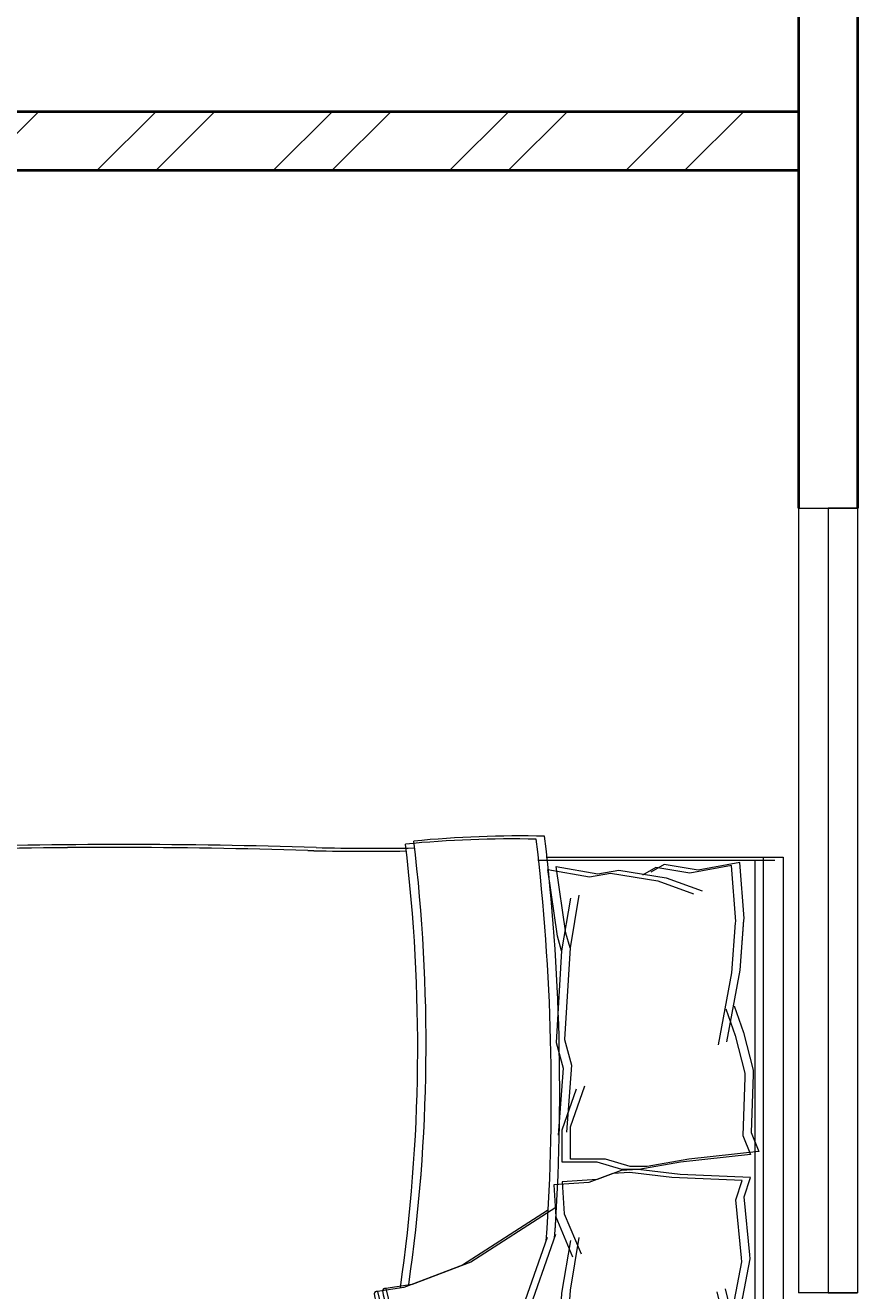
# Model space of a CAD drawing. Units: inches. Extents: x 1601 to 2297, y 1496 to 2631.
# Tile 48 of 57: x 2167 to 2231, y 2141 to 2237. Entities that reach past the tile are written whole.
import ezdxf

# ---------------------------------------------------------------- set-up
doc = ezdxf.new("R2010")
doc.units = ezdxf.units.IN
for name, color, linetype, lineweight in [('A-ANNO-DIMS', 2, 'Continuous', 18), ('A-FURN', 8, 'Continuous', 18), ('A-GLAZ', 161, 'Continuous', 20), ('A-WALL', 7, 'Continuous', 40), ('A-WALL-PATT', 215, 'Continuous', 13)]:
    doc.layers.add(name, color=color, linetype=linetype, lineweight=lineweight)
doc.styles.get("Standard").update_dxf_attribs({"font": 'arial.ttf'})
doc.dimstyles.get("Standard").update_dxf_attribs({"dimtxt": 0.18, "dimasz": 0.18, "dimexe": 0.18, "dimexo": 0.0625, "dimgap": 0.09, "dimtad": 0, "dimtih": 1, "dimtoh": 1, "dimdec": 4, "dimzin": 0, "dimdsep": 46, "dimtxsty": 'Standard', "dimcen": 0.09, "dimadec": 0, "dimazin": 0, "dimtfac": 1, "dimtdec": 4, "dimtofl": 0, "dimtmove": 0, "dimatfit": 3, "dimfxl": 1, "dimtolj": 1, "dimtzin": 0, "dimarcsym": 0})

# ---------------------------------------------------------------- blocks, each defined once
blk = doc.blocks.new('BED-DOUBLE')
for p, q in [((27.746, 52.867), (24.495, 49.162)), ((27.746, 52.867), (24.495, 49.162)), ((27.746, 52.867), (24.495, 49.162)), ((27.746, 52.867), (24.495, 49.162)), ((28.385, 53.096), (25.135, 49.39)), ((28.385, 53.096), (25.135, 49.39)), ((28.385, 53.096), (25.135, 49.39)), ((28.385, 53.096), (25.135, 49.39)), ((29.49, 52.947), (27.746, 52.867, 3.871)), ((29.49, 52.947), (27.746, 52.867, 3.871)), ((29.49, 52.947), (27.746, 52.867, 3.871)), ((29.49, 52.947), (27.746, 52.867, 3.871)), ((28.365, 51.33), (27.746, 52.867)), ((28.365, 51.33), (27.746, 52.867)), ((28.365, 51.33), (27.746, 52.867)), ((28.365, 51.33), (27.746, 52.867)), ((30.13, 53.175), (28.385, 53.096, 3.871)), ((30.13, 53.175), (28.385, 53.096, 3.871)), ((30.13, 53.175), (28.385, 53.096, 3.871)), ((30.13, 53.175), (28.385, 53.096, 3.871)), ((29.004, 51.559), (28.385, 53.096)), ((29.004, 51.558), (28.385, 53.096)), ((29.004, 51.559), (28.385, 53.096)), ((29.004, 51.558), (28.385, 53.096)), ((0, 51.494), (0.639, 51.493)), ((0, 3.475), (0, 51.494)), ((0, 51.494), (0.639, 51.493)), ((0, 3.475), (0, 51.494)), ((0.639, 51.494), (27.249, 51.494)), ((0.639, 51.494), (27.249, 51.494)), ((0.639, 51.493), (27.249, 51.493)), ((0.639, 51.493), (27.249, 51.493)), ((2.173, 3.703), (2.173, 51.494)), ((2.173, 3.703), (2.173, 51.494)), ((2.173, 3.703), (2.173, 51.493)), ((2.173, 3.703), (2.173, 51.493)), ((28.055, 48.233), (28.365, 51.33)), ((28.055, 48.233), (28.365, 51.33)), ((28.055, 48.233), (28.365, 51.33)), ((28.055, 48.233), (28.365, 51.33)), ((28.695, 48.461), (29.004, 51.559)), ((28.695, 48.461), (29.004, 51.559)), ((28.695, 48.461), (29.004, 51.558)), ((28.695, 48.461), (29.004, 51.558)), ((0, 51.265), (26.61, 51.265)), ((0, 51.265), (26.61, 51.265)), ((0, 51.265), (26.61, 51.265)), ((0, 51.265), (26.61, 51.265)), ((1.533, 3.475), (1.533, 51.265)), ((1.533, 3.475), (1.533, 51.265)), ((1.533, 3.475), (1.533, 51.265)), ((1.533, 3.475), (1.533, 51.265)), ((3.196, 50.34), (3.099, 44.938)), ((3.196, 50.34), (3.099, 44.938)), ((3.196, 50.34), (3.099, 44.938)), ((3.196, 50.34), (3.099, 44.938)), ((3.196, 50.34), (6.407, 49.961)), ((3.196, 50.34), (6.407, 49.961)), ((3.196, 50.34), (6.407, 49.961)), ((3.196, 50.34), (6.407, 49.961)), ((5.768, 49.733), (8.338, 50.328)), ((5.768, 49.733), (8.338, 50.328)), ((5.768, 49.733), (8.338, 50.328)), ((5.768, 49.733), (8.338, 50.328)), ((6.407, 49.961), (8.977, 50.557)), ((6.407, 49.961), (8.977, 50.557)), ((6.407, 49.961), (8.977, 50.556)), ((6.407, 49.961), (8.977, 50.556)), ((8.338, 50.328), (9.384, 49.814)), ((8.338, 50.328), (9.384, 49.814)), ((8.338, 50.328), (9.384, 49.814)), ((8.338, 50.328), (9.384, 49.814)), ((12.468, 50.34), (8.896, 49.538)), ((12.468, 50.34), (8.896, 49.537)), ((12.468, 50.34), (8.896, 49.538)), ((12.468, 50.34), (8.896, 49.537)), ((8.977, 50.557), (10.024, 50.043)), ((8.977, 50.557), (10.024, 50.043)), ((8.977, 50.556), (10.024, 50.042)), ((8.977, 50.556), (10.024, 50.042)), ((14.073, 50.151), (12.468, 50.34)), ((14.073, 50.151), (12.468, 50.34)), ((14.073, 50.151), (12.468, 50.34)), ((14.073, 50.151), (12.468, 50.34)), ((16.573, 50.698), (13.434, 49.923)), ((16.573, 50.698), (13.434, 49.922)), ((16.573, 50.698), (13.434, 49.923)), ((16.573, 50.698), (13.434, 49.922)), ((17.212, 50.926), (14.073, 50.151)), ((17.212, 50.926), (14.073, 50.151)), ((17.212, 50.926), (14.073, 50.151)), ((17.212, 50.926), (14.073, 50.151)), ((16.169, 45.566), (16.573, 50.698)), ((16.169, 45.566), (16.573, 50.698)), ((16.169, 45.566), (16.573, 50.698)), ((16.169, 45.566), (16.573, 50.698)), ((16.808, 45.795), (17.212, 50.926)), ((16.808, 45.794), (17.212, 50.926)), ((16.808, 45.795), (17.212, 50.926)), ((16.808, 45.794), (17.212, 50.926)), ((2.557, 50.112), (2.46, 44.709)), ((2.557, 50.112), (2.46, 44.709)), ((2.557, 50.111), (2.46, 44.709)), ((2.557, 50.111), (2.46, 44.709)), ((2.557, 50.112), (5.768, 49.733)), ((2.557, 50.112), (5.768, 49.733)), ((2.557, 50.111), (5.768, 49.733)), ((2.557, 50.111), (5.768, 49.733)), ((8.896, 49.538), (6.218, 48.356)), ((8.896, 49.538), (6.218, 48.356)), ((8.896, 49.537), (6.218, 48.356)), ((8.896, 49.537), (6.218, 48.356)), ((11.829, 50.112), (8.257, 49.309)), ((11.829, 50.112), (8.257, 49.309)), ((11.829, 50.112), (8.257, 49.309)), ((11.829, 50.112), (8.257, 49.309)), ((13.434, 49.923), (11.829, 50.112)), ((13.434, 49.922), (11.829, 50.112)), ((13.434, 49.923), (11.829, 50.112)), ((13.434, 49.922), (11.829, 50.112)), ((25.135, 49.39), (22.968, 46.448)), ((25.135, 49.39), (22.968, 46.448)), ((25.135, 49.39), (22.968, 46.448)), ((25.135, 49.39), (22.968, 46.448)), ((8.257, 49.309), (5.578, 48.128)), ((8.257, 49.309), (5.578, 48.128)), ((8.257, 49.309), (5.578, 48.128)), ((8.257, 49.309), (5.578, 48.128)), ((24.495, 49.162), (22.329, 46.219)), ((24.495, 49.162), (22.329, 46.219)), ((24.495, 49.162), (22.329, 46.219)), ((24.495, 49.162), (22.329, 46.219)), ((29.004, 44.589), (28.695, 48.461)), ((29.004, 44.589), (28.695, 48.461)), ((29.004, 44.589), (28.695, 48.461)), ((29.004, 44.589), (28.695, 48.461)), ((28.365, 44.361), (28.055, 48.233)), ((28.365, 44.361), (28.055, 48.233)), ((28.365, 44.361), (28.055, 48.233)), ((28.365, 44.361), (28.055, 48.233)), ((22.968, 46.448), (20.956, 40.872)), ((22.968, 46.448), (20.956, 40.872)), ((22.968, 46.448), (20.956, 40.872)), ((22.968, 46.448), (20.956, 40.872)), ((2.46, 44.709), (2.542, 45.712)), ((2.46, 44.709), (2.542, 45.712)), ((2.46, 44.709), (2.542, 45.712)), ((2.46, 44.709), (2.542, 45.712)), ((2.542, 45.712), (3.069, 41.914)), ((2.542, 45.712), (3.069, 41.914)), ((2.542, 45.712), (3.069, 41.914)), ((2.542, 45.712), (3.069, 41.914)), ((3.099, 44.938), (3.181, 45.941)), ((3.099, 44.938), (3.181, 45.941)), ((3.099, 44.938), (3.181, 45.94)), ((3.099, 44.938), (3.181, 45.94)), ((3.181, 45.941), (3.709, 42.143)), ((3.181, 45.941), (3.709, 42.143)), ((3.181, 45.94), (3.709, 42.142)), ((3.181, 45.94), (3.709, 42.142)), ((16.726, 43.606), (16.169, 45.566)), ((16.726, 43.606), (16.169, 45.566)), ((16.726, 43.606), (16.169, 45.566)), ((16.726, 43.606), (16.169, 45.566)), ((17.365, 43.834), (16.808, 45.795)), ((17.365, 43.834), (16.808, 45.795)), ((17.365, 43.834), (16.808, 45.794)), ((17.365, 43.834), (16.808, 45.794)), ((22.329, 46.219), (20.316, 40.644)), ((22.329, 46.219), (20.316, 40.644)), ((22.329, 46.219), (20.317, 40.644)), ((22.329, 46.219), (20.317, 40.644)), ((29.468, 41.182), (29.004, 44.589)), ((29.469, 41.182), (29.004, 44.589)), ((29.468, 41.182), (29.004, 44.589)), ((29.469, 41.182), (29.004, 44.589)), ((16.295, 36.596), (16.726, 43.606)), ((16.295, 36.596), (16.726, 43.606)), ((16.295, 36.596), (16.726, 43.606)), ((16.295, 36.596), (16.726, 43.606)), ((16.934, 36.824), (17.365, 43.834)), ((16.934, 36.824), (17.365, 43.834)), ((16.934, 36.824), (17.365, 43.834)), ((16.934, 36.824), (17.365, 43.834)), ((28.829, 40.954), (28.365, 44.361)), ((28.829, 40.953), (28.365, 44.361)), ((28.829, 40.954), (28.365, 44.361)), ((28.829, 40.953), (28.365, 44.361)), ((3.069, 41.914), (4.422, 36.495)), ((3.069, 41.914), (4.422, 36.495)), ((3.069, 41.914), (4.422, 36.495)), ((3.069, 41.914), (4.422, 36.495)), ((3.709, 42.143), (5.061, 36.723)), ((3.709, 42.143), (5.061, 36.723)), ((3.709, 42.142), (5.061, 36.723)), ((3.709, 42.142), (5.061, 36.723)), ((20.316, 40.644), (17.383, 32.306)), ((20.317, 40.644), (17.383, 32.306)), ((20.316, 40.644), (17.383, 32.306)), ((20.317, 40.644), (17.383, 32.306)), ((20.956, 40.872), (18.022, 32.534)), ((20.956, 40.872), (18.022, 32.534)), ((20.956, 40.872), (18.022, 32.534)), ((20.956, 40.872), (18.022, 32.534)), ((29.758, 38.94), (28.829, 40.954)), ((29.758, 38.94), (28.829, 40.954)), ((29.758, 38.94), (28.829, 40.953)), ((29.758, 38.94), (28.829, 40.953)), ((30.397, 39.169), (29.468, 41.182)), ((30.397, 39.169), (29.468, 41.182)), ((30.397, 39.168), (29.469, 41.182)), ((30.397, 39.168), (29.469, 41.182)), ((79.245, 15.063), (79.245, 39.677)), ((79.245, 15.063), (79.245, 39.677)), ((79.245, 15.063), (79.245, 39.677)), ((79.245, 15.063), (79.245, 39.677)), ((79.884, 15.292), (79.884, 39.905)), ((79.884, 15.291), (79.884, 39.905)), ((79.884, 15.292), (79.884, 39.905)), ((79.884, 15.291), (79.884, 39.905)), ((3.673, 39.2), (3.078, 37.135)), ((3.673, 39.2), (3.078, 37.135)), ((3.673, 39.2), (3.078, 37.135)), ((3.673, 39.2), (3.078, 37.135)), ((4.313, 39.428), (3.717, 37.363)), ((4.313, 39.428), (3.717, 37.363)), ((4.313, 39.428), (3.718, 37.363)), ((4.313, 39.428), (3.718, 37.363)), ((30.377, 36.462), (29.758, 38.94)), ((30.377, 36.462), (29.758, 38.94)), ((30.377, 36.462), (29.758, 38.94)), ((30.377, 36.462), (29.758, 38.94)), ((31.016, 36.691), (30.397, 39.169)), ((31.016, 36.691), (30.397, 39.169)), ((31.016, 36.691), (30.397, 39.168)), ((31.016, 36.691), (30.397, 39.168)), ((3.078, 37.135), (2.537, 34.204)), ((3.078, 37.135), (2.537, 34.204)), ((3.078, 37.135), (2.537, 34.204)), ((3.078, 37.135), (2.537, 34.204)), ((3.717, 37.363), (3.176, 34.433)), ((3.718, 37.363), (3.176, 34.433)), ((3.717, 37.363), (3.176, 34.433)), ((3.718, 37.363), (3.176, 34.433)), ((16.268, 32.792), (16.934, 36.824)), ((16.268, 32.792), (16.934, 36.824)), ((16.268, 32.792), (16.934, 36.824)), ((16.268, 32.792), (16.934, 36.824)), ((15.628, 32.564), (16.295, 36.596)), ((15.628, 32.564), (16.295, 36.596)), ((15.628, 32.564), (16.295, 36.596)), ((15.628, 32.564), (16.295, 36.596)), ((23.876, 34.449), (28.365, 36.153)), ((23.876, 34.449), (28.365, 36.153)), ((23.876, 34.449), (28.365, 36.152)), ((23.876, 34.449), (28.365, 36.152)), ((24.516, 34.677), (29.004, 36.381)), ((24.516, 34.677), (29.004, 36.381)), ((24.516, 34.677), (29.004, 36.381)), ((24.516, 34.677), (29.004, 36.381)), ((28.365, 36.153), (30.377, 36.462)), ((28.365, 36.152), (30.377, 36.462)), ((28.365, 36.153), (30.377, 36.462)), ((28.365, 36.152), (30.377, 36.462)), ((29.004, 36.381), (31.016, 36.691)), ((29.004, 36.381), (31.016, 36.691)), ((29.004, 36.381), (31.016, 36.691)), ((29.004, 36.381), (31.016, 36.691)), ((2.537, 34.204), (2.557, 33.883)), ((2.537, 34.204), (2.557, 33.883)), ((2.537, 34.204), (2.557, 33.883)), ((2.537, 34.204), (2.557, 33.883)), ((2.557, 33.883), (2.979, 29.456)), ((2.557, 33.883), (2.979, 29.455)), ((2.557, 33.883), (2.979, 29.456)), ((2.557, 33.883), (2.979, 29.455)), ((3.176, 34.433), (3.196, 34.112)), ((3.176, 34.433), (3.196, 34.112)), ((3.176, 34.433), (3.196, 34.112)), ((3.176, 34.433), (3.196, 34.112)), ((3.196, 34.112), (3.618, 29.684)), ((3.196, 34.112), (3.618, 29.684)), ((3.196, 34.112), (3.618, 29.684)), ((3.196, 34.112), (3.618, 29.684)), ((17.379, 30.978), (16.094, 34.049)), ((17.379, 30.978), (16.094, 34.049)), ((17.379, 30.978), (16.094, 34.049)), ((17.379, 30.978), (16.094, 34.049)), ((17.383, 30.259), (23.876, 34.449)), ((17.383, 30.259), (23.876, 34.449)), ((17.383, 30.259), (23.876, 34.449)), ((17.383, 30.259), (23.876, 34.449)), ((18.022, 30.487), (24.516, 34.677)), ((18.022, 30.487), (24.516, 34.677)), ((18.022, 30.487), (24.516, 34.677)), ((18.022, 30.487), (24.516, 34.677)), ((16.739, 30.75), (15.454, 33.821)), ((16.739, 30.75), (15.454, 33.821)), ((16.739, 30.75), (15.454, 33.82)), ((16.739, 30.75), (15.454, 33.82)), ((17.532, 28.526), (17.379, 30.978)), ((17.532, 28.525), (17.379, 30.978)), ((17.532, 28.526), (17.379, 30.978)), ((17.532, 28.525), (17.379, 30.978)), ((16.893, 28.297), (16.739, 30.75)), ((16.893, 28.297), (16.739, 30.75)), ((16.893, 28.297), (16.739, 30.75)), ((16.893, 28.297), (16.739, 30.75)), ((2.979, 29.456), (2.492, 27.977)), ((2.979, 29.456), (2.492, 27.977)), ((2.979, 29.455), (2.492, 27.976)), ((2.979, 29.455), (2.492, 27.976)), ((3.618, 29.684), (3.131, 28.205)), ((3.618, 29.684), (3.131, 28.205)), ((3.618, 29.684), (3.131, 28.205)), ((3.618, 29.684), (3.131, 28.205)), ((3.131, 28.205), (8.506, 27.962)), ((3.131, 28.205), (8.506, 27.961)), ((3.131, 28.205), (8.506, 27.962)), ((3.131, 28.205), (8.506, 27.961)), ((12.377, 27.436), (14.216, 28.13)), ((12.377, 27.436), (14.217, 28.13)), ((12.377, 27.436), (14.216, 28.13)), ((12.377, 27.436), (14.217, 28.13)), ((13.016, 27.664), (14.856, 28.359)), ((13.016, 27.664), (14.856, 28.359)), ((13.016, 27.664), (14.856, 28.358)), ((13.016, 27.664), (14.856, 28.358)), ((14.216, 28.13), (16.893, 28.297)), ((14.216, 28.13), (16.893, 28.297)), ((14.217, 28.13), (16.893, 28.297)), ((14.217, 28.13), (16.893, 28.297)), ((14.856, 28.359), (17.532, 28.526)), ((14.856, 28.359), (17.532, 28.526)), ((14.856, 28.358), (17.532, 28.525)), ((14.856, 28.358), (17.532, 28.525)), ((2.492, 27.977), (7.867, 27.733)), ((2.492, 27.977), (7.867, 27.733)), ((2.492, 27.976), (7.867, 27.733)), ((2.492, 27.976), (7.867, 27.733)), ((7.22, 26.561), (10.401, 27.139)), ((7.22, 26.56), (10.401, 27.139)), ((7.22, 26.561), (10.401, 27.139)), ((7.22, 26.56), (10.401, 27.139)), ((7.859, 26.789), (11.04, 27.367)), ((7.859, 26.789), (11.04, 27.367)), ((7.859, 26.789), (11.04, 27.367)), ((7.859, 26.789), (11.04, 27.367)), ((7.867, 27.733), (11.078, 27.355)), ((7.867, 27.733), (11.078, 27.354)), ((7.867, 27.733), (11.078, 27.355)), ((7.867, 27.733), (11.078, 27.354)), ((8.506, 27.962), (11.717, 27.583)), ((8.506, 27.962), (11.717, 27.583)), ((8.506, 27.961), (11.717, 27.583)), ((8.506, 27.961), (11.717, 27.583)), ((10.401, 27.139), (11.702, 27.139)), ((10.401, 27.139), (11.702, 27.139)), ((10.401, 27.139), (11.702, 27.139)), ((10.401, 27.139), (11.702, 27.139)), ((11.04, 27.367), (12.341, 27.367)), ((11.04, 27.367), (12.341, 27.367)), ((11.04, 27.367), (12.341, 27.367)), ((11.04, 27.367), (12.341, 27.367)), ((11.078, 27.355), (12.377, 27.436)), ((11.078, 27.354), (12.377, 27.436)), ((11.078, 27.355), (12.377, 27.436)), ((11.078, 27.354), (12.377, 27.436)), ((11.702, 27.139), (13.582, 26.561)), ((11.702, 27.139), (13.582, 26.56)), ((11.702, 27.139), (13.582, 26.561)), ((11.702, 27.139), (13.582, 26.56)), ((11.717, 27.583), (13.016, 27.664)), ((11.717, 27.583), (13.016, 27.664)), ((11.717, 27.583), (13.016, 27.664)), ((11.717, 27.583), (13.016, 27.664)), ((12.341, 27.367), (14.221, 26.789)), ((12.341, 27.367), (14.221, 26.789)), ((12.341, 27.367), (14.221, 26.789)), ((12.341, 27.367), (14.221, 26.789)), ((1.87, 25.982), (7.22, 26.561)), ((1.87, 25.982), (7.22, 26.561)), ((1.87, 25.982), (7.22, 26.56)), ((1.87, 25.982), (7.22, 26.56)), ((2.509, 26.211), (7.859, 26.789)), ((2.509, 26.21), (7.859, 26.789)), ((2.509, 26.211), (7.859, 26.789)), ((2.509, 26.21), (7.859, 26.789)), ((3.088, 24.765), (2.509, 26.211)), ((3.088, 24.765), (2.509, 26.211)), ((3.088, 24.765), (2.509, 26.21)), ((3.088, 24.765), (2.509, 26.21)), ((13.582, 26.561), (16.263, 26.561)), ((13.582, 26.561), (16.263, 26.561)), ((13.582, 26.56), (16.263, 26.56)), ((13.582, 26.56), (16.263, 26.56)), ((14.221, 26.789), (16.902, 26.789)), ((14.221, 26.789), (16.902, 26.789)), ((14.221, 26.789), (16.902, 26.789)), ((14.221, 26.789), (16.902, 26.789)), ((16.263, 26.561), (16.263, 24.103)), ((16.263, 26.561), (16.263, 24.103)), ((16.263, 26.56), (16.263, 24.103)), ((16.263, 26.56), (16.263, 24.103)), ((16.902, 26.789), (16.902, 24.332)), ((16.902, 26.789), (16.902, 24.331)), ((16.902, 26.789), (16.902, 24.332)), ((16.902, 26.789), (16.902, 24.331)), ((2.448, 24.537), (1.87, 25.982)), ((2.448, 24.537), (1.87, 25.982)), ((2.448, 24.537), (1.87, 25.982)), ((2.448, 24.537), (1.87, 25.982)), ((2.304, 20.091), (2.448, 24.537)), ((2.304, 20.091), (2.448, 24.537)), ((2.304, 20.091), (2.448, 24.537)), ((2.304, 20.091), (2.448, 24.537)), ((2.943, 20.32), (3.088, 24.765)), ((2.943, 20.319), (3.088, 24.765)), ((2.943, 20.32), (3.088, 24.765)), ((2.943, 20.319), (3.088, 24.765)), ((16.902, 24.332), (15.811, 21.187)), ((16.902, 24.332), (15.811, 21.187)), ((16.902, 24.331), (15.811, 21.187)), ((16.902, 24.331), (15.811, 21.187)), ((16.169, 19.384), (16.573, 24.516)), ((16.169, 19.384), (16.573, 24.516)), ((16.169, 19.383), (16.573, 24.515)), ((16.169, 19.383), (16.573, 24.515)), ((16.808, 19.612), (17.212, 24.744)), ((16.808, 19.612), (17.212, 24.744)), ((16.808, 19.612), (17.212, 24.744)), ((16.808, 19.612), (17.212, 24.744)), ((16.263, 24.103), (15.172, 20.959)), ((16.263, 24.103), (15.172, 20.958)), ((16.263, 24.103), (15.172, 20.959)), ((16.263, 24.103), (15.172, 20.958)), ((2.943, 19.998), (2.943, 20.32)), ((2.943, 19.998), (2.943, 20.32)), ((2.943, 19.998), (2.943, 20.319)), ((2.943, 19.998), (2.943, 20.319)), ((2.304, 19.77), (2.304, 20.091)), ((2.304, 19.769), (2.304, 20.091)), ((2.304, 19.77), (2.304, 20.091)), ((2.304, 19.769), (2.304, 20.091)), ((3.027, 16.878), (2.304, 19.77)), ((3.027, 16.878), (2.304, 19.77)), ((3.027, 16.878), (2.304, 19.769)), ((3.027, 16.878), (2.304, 19.769)), ((3.666, 17.107), (2.943, 19.998)), ((3.666, 17.107), (2.943, 19.998)), ((3.666, 17.107), (2.943, 19.998)), ((3.666, 17.107), (2.943, 19.998)), ((16.726, 17.423), (16.169, 19.384)), ((16.726, 17.423), (16.169, 19.384)), ((16.726, 17.423), (16.169, 19.383)), ((16.726, 17.423), (16.169, 19.383)), ((17.365, 17.652), (16.808, 19.612)), ((17.365, 17.651), (16.808, 19.612)), ((17.365, 17.652), (16.808, 19.612)), ((17.365, 17.651), (16.808, 19.612)), ((3.316, 12.108), (4.328, 17.601)), ((3.316, 12.108), (4.328, 17.601)), ((3.316, 12.108), (4.328, 17.601)), ((3.316, 12.108), (4.328, 17.601)), ((3.955, 12.336), (4.967, 17.83)), ((3.955, 12.336), (4.967, 17.83)), ((3.955, 12.336), (4.967, 17.829)), ((3.955, 12.336), (4.967, 17.829)), ((16.295, 10.413), (16.726, 17.423)), ((16.295, 10.413), (16.726, 17.423)), ((16.295, 10.413), (16.726, 17.423)), ((16.295, 10.413), (16.726, 17.423)), ((16.934, 10.642), (17.365, 17.652)), ((16.934, 10.642), (17.365, 17.652)), ((16.934, 10.642), (17.365, 17.651)), ((16.934, 10.642), (17.365, 17.651)), ((3.75, 14.855), (3.027, 16.878)), ((3.75, 14.854), (3.027, 16.878)), ((3.75, 14.855), (3.027, 16.878)), ((3.75, 14.854), (3.027, 16.878)), ((4.389, 15.083), (3.666, 17.107)), ((4.389, 15.083), (3.666, 17.107)), ((4.389, 15.083), (3.666, 17.107)), ((4.389, 15.083), (3.666, 17.107)), ((3.027, 8.285), (3.316, 12.108)), ((3.027, 8.284), (3.316, 12.108)), ((3.027, 8.285), (3.316, 12.108)), ((3.027, 8.284), (3.316, 12.108)), ((3.666, 8.513), (3.955, 12.336)), ((3.666, 8.513), (3.955, 12.336)), ((3.666, 8.513), (3.955, 12.336)), ((3.666, 8.513), (3.955, 12.336)), ((15.628, 6.382), (16.295, 10.413)), ((15.628, 6.381), (16.295, 10.413)), ((15.628, 6.382), (16.295, 10.413)), ((15.628, 6.381), (16.295, 10.413)), ((16.268, 6.61), (16.934, 10.642)), ((16.268, 6.61), (16.934, 10.642)), ((16.268, 6.61), (16.934, 10.642)), ((16.268, 6.61), (16.934, 10.642)), ((16.295, 10.413), (16.618, 9.28)), ((16.295, 10.413), (16.618, 9.28)), ((16.295, 10.413), (16.618, 9.28)), ((16.295, 10.413), (16.618, 9.28)), ((16.934, 10.642), (17.257, 9.509)), ((16.934, 10.642), (17.257, 9.508)), ((16.934, 10.642), (17.257, 9.509)), ((16.934, 10.642), (17.257, 9.508)), ((16.618, 9.28), (17.341, 4.184)), ((16.618, 9.28), (17.341, 4.183)), ((16.618, 9.28), (17.341, 4.184)), ((16.618, 9.28), (17.341, 4.183)), ((17.257, 9.509), (17.98, 4.412)), ((17.257, 9.509), (17.98, 4.412)), ((17.257, 9.508), (17.98, 4.412)), ((17.257, 9.508), (17.98, 4.412)), ((3.009, 8.179), (3.027, 8.285)), ((3.009, 8.179), (3.027, 8.285)), ((3.009, 8.179), (3.027, 8.284)), ((3.009, 8.179), (3.027, 8.284)), ((3.338, 3.898), (3.009, 8.179)), ((3.338, 3.898), (3.009, 8.179)), ((3.338, 3.898), (3.009, 8.179)), ((3.338, 3.898), (3.009, 8.179)), ((3.648, 8.408), (3.666, 8.513)), ((3.648, 8.407), (3.666, 8.513)), ((3.648, 8.408), (3.666, 8.513)), ((3.648, 8.407), (3.666, 8.513)), ((3.977, 4.127), (3.648, 8.408)), ((3.977, 4.127), (3.648, 8.408)), ((3.977, 4.127), (3.648, 8.407)), ((3.977, 4.127), (3.648, 8.407)), ((8.955, 5.051), (6.208, 6.063)), ((8.955, 5.051), (6.208, 6.063)), ((8.955, 5.051), (6.208, 6.063)), ((8.955, 5.051), (6.208, 6.063)), ((9.594, 5.279), (6.847, 6.291)), ((9.594, 5.279), (6.847, 6.291)), ((9.594, 5.279), (6.847, 6.291)), ((9.594, 5.279), (6.847, 6.291)), ((12.57, 4.473), (8.955, 5.051)), ((12.57, 4.472), (8.955, 5.051)), ((12.57, 4.473), (8.955, 5.051)), ((12.57, 4.472), (8.955, 5.051)), ((13.209, 4.701), (9.594, 5.279)), ((13.209, 4.701), (9.594, 5.279)), ((13.209, 4.701), (9.594, 5.279)), ((13.209, 4.701), (9.594, 5.279)), ((9.739, 4.267), (10.751, 4.846)), ((9.739, 4.267), (10.751, 4.846)), ((9.739, 4.267), (10.751, 4.845)), ((9.739, 4.267), (10.751, 4.845)), ((14.799, 4.99), (13.209, 4.701)), ((14.799, 4.99), (13.209, 4.701)), ((14.799, 4.99), (13.209, 4.701)), ((14.799, 4.99), (13.209, 4.701)), ((17.98, 4.412), (14.799, 4.99)), ((17.98, 4.412), (14.799, 4.99)), ((17.98, 4.412), (14.799, 4.99)), ((17.98, 4.412), (14.799, 4.99)), ((3.316, 3.894), (6.497, 4.473)), ((3.316, 3.894), (6.497, 4.473)), ((3.316, 3.894), (6.497, 4.472)), ((3.316, 3.894), (6.497, 4.472)), ((3.955, 4.123), (7.136, 4.701)), ((3.955, 4.123), (7.136, 4.701)), ((3.955, 4.123), (7.136, 4.701)), ((3.955, 4.123), (7.136, 4.701)), ((6.497, 4.473), (9.099, 4.039)), ((6.497, 4.473), (9.099, 4.039)), ((6.497, 4.472), (9.099, 4.039)), ((6.497, 4.472), (9.099, 4.039)), ((7.136, 4.701), (9.739, 4.267)), ((7.136, 4.701), (9.739, 4.267)), ((7.136, 4.701), (9.739, 4.267)), ((7.136, 4.701), (9.739, 4.267)), ((9.099, 4.039), (10.112, 4.617)), ((9.099, 4.039), (10.112, 4.617)), ((9.099, 4.039), (10.112, 4.617)), ((9.099, 4.039), (10.112, 4.617)), ((14.16, 4.762), (12.57, 4.473)), ((14.16, 4.762), (12.57, 4.472)), ((14.16, 4.762), (12.57, 4.473)), ((14.16, 4.762), (12.57, 4.472)), ((17.341, 4.184), (14.16, 4.762)), ((17.341, 4.183), (14.16, 4.762)), ((17.341, 4.184), (14.16, 4.762)), ((17.341, 4.183), (14.16, 4.762)), ((18.11, 3.475), (0, 3.475)), ((18.11, 3.475), (0, 3.475)), ((18.11, 3.475), (0, 3.475)), ((18.11, 3.475), (0, 3.475)), ((18.75, 3.703), (0.639, 3.703)), ((18.75, 3.703), (0.639, 3.703)), ((18.75, 3.703), (0.639, 3.703)), ((18.75, 3.703), (0.639, 3.703))]:
    blk.add_line(p, q)
for centre, radius, start, end in [((68.666, 76.157), 23.065, 267.47136, 296.46809), ((68.666, 76.157), 23.065, 267.47136, 296.46809), ((68.666, 76.157), 23.065, 267.47136, 296.46809), ((68.666, 76.157), 23.065, 267.47136, 296.46809), ((69.306, 76.385), 23.065, 267.47136, 296.46809), ((69.306, 76.385), 23.065, 267.47136, 296.46809), ((69.306, 76.385), 23.065, 267.47136, 296.46809), ((69.306, 76.385), 23.065, 267.47136, 296.46809), ((78.87, 54.41), 1.102, 332.65876, 86.02002), ((78.87, 54.409), 1.102, 332.65876, 86.02002), ((78.87, 54.41), 1.102, 332.65876, 86.02002), ((78.87, 54.409), 1.102, 332.65876, 86.02002), ((79.509, 54.638), 1.102, 332.65876, 86.02002), ((79.509, 54.638), 1.102, 332.65876, 86.02002), ((79.509, 54.638), 1.102, 332.65876, 86.02002), ((79.509, 54.638), 1.102, 332.65876, 86.02002), ((36.954, 182.494), 129.499, 266.97912, 273.83645), ((36.954, 182.494), 129.499, 266.97912, 273.83645), ((36.954, 182.494), 129.499, 266.97912, 273.83645), ((36.954, 182.494), 129.499, 266.97912, 273.83645), ((68.461, -4508.515), 4561.858, 90.002168, 90.286887), ((68.461, -4508.515), 4561.858, 90.002168, 90.286887), ((68.461, -4508.516), 4561.858, 90.002168, 90.286887), ((68.461, -4508.516), 4561.858, 90.002168, 90.286887), ((212.276, 41.152), 133.04, 174.4998, 180.63509), ((212.277, 41.151), 133.04, 174.4998, 180.63509), ((212.276, 41.152), 133.04, 174.4998, 180.63509), ((212.277, 41.151), 133.04, 174.4998, 180.63509), ((212.916, 41.38), 133.04, 174.4998, 180.63509), ((212.916, 41.38), 133.04, 174.4998, 180.63509), ((212.916, 41.38), 133.04, 174.4998, 180.63509), ((212.916, 41.38), 133.04, 174.4998, 180.63509), ((-6.656, 51.327), 36.183, 349.87628, 2.56571), ((-6.656, 51.327), 36.183, 349.87628, 2.56571), ((-6.656, 51.327), 36.183, 349.87628, 2.56571), ((-6.656, 51.327), 36.183, 349.87628, 2.56571), ((36.315, 182.266), 129.499, 266.97912, 273.83645), ((36.315, 182.265), 129.499, 266.97912, 273.83645), ((36.315, 182.266), 129.499, 266.97912, 273.83645), ((36.315, 182.265), 129.499, 266.97912, 273.83645), ((-6.017, 51.555), 36.183, 349.87628, 2.56571), ((-6.017, 51.555), 36.183, 349.87628, 2.56571), ((-6.017, 51.555), 36.183, 349.87628, 2.56571), ((-6.017, 51.555), 36.183, 349.87628, 2.56571), ((67.821, -4508.744), 4561.858, 90.002168, 90.286887), ((67.821, -4508.744), 4561.858, 90.002168, 90.286887), ((67.821, -4508.744), 4561.858, 90.002168, 90.286887), ((67.821, -4508.744), 4561.858, 90.002168, 90.286887), ((35.066, 43.743), 6.224, 168.6608, 203.73842), ((35.066, 43.743), 6.224, 168.6608, 203.73842), ((35.066, 43.743), 6.224, 168.6608, 203.73842), ((35.066, 43.743), 6.224, 168.6608, 203.73842), ((35.705, 43.972), 6.224, 168.6608, 203.73842), ((35.705, 43.971), 6.224, 168.6608, 203.73842), ((35.705, 43.972), 6.224, 168.6608, 203.73842), ((35.705, 43.971), 6.224, 168.6608, 203.73842), ((1.482, 31.154), 29.654, 10.66171, 19.88058), ((1.482, 31.154), 29.654, 10.66171, 19.88058), ((1.482, 31.153), 29.654, 10.66171, 19.88058), ((1.482, 31.153), 29.654, 10.66171, 19.88058), ((2.121, 31.382), 29.654, 10.66171, 19.88058), ((2.121, 31.382), 29.654, 10.66171, 19.88058), ((2.121, 31.382), 29.654, 10.66171, 19.88058), ((2.121, 31.382), 29.654, 10.66171, 19.88058), ((31.079, 36.864), 0.185, 250.24637, 1.13765), ((31.079, 36.864), 0.185, 250.24637, 1.13765), ((31.079, 36.864), 0.185, 250.24637, 1.13765), ((31.079, 36.864), 0.185, 250.24637, 1.13765), ((156.316, 17.756), 129.02, 171.78449, 186.90062), ((156.316, 17.755), 129.02, 171.78449, 186.90062), ((156.316, 17.756), 129.02, 171.78449, 186.90062), ((156.316, 17.755), 129.02, 171.78449, 186.90062), ((156.955, 17.984), 129.02, 171.78449, 186.90062), ((156.955, 17.984), 129.02, 171.78449, 186.90062), ((156.955, 17.984), 129.02, 171.78449, 186.90062), ((156.955, 17.984), 129.02, 171.78449, 186.90062), ((30.439, 36.636), 0.185, 250.24637, 1.13765), ((30.439, 36.636), 0.185, 250.24637, 1.13765), ((30.439, 36.636), 0.185, 250.24637, 1.13765), ((30.439, 36.636), 0.185, 250.24637, 1.13765), ((182.052, 21.359), 164.969, 176.08655, 186.78213), ((182.052, 21.359), 164.969, 176.08655, 186.78213), ((182.052, 21.358), 164.969, 176.08655, 186.78213), ((182.052, 21.358), 164.969, 176.08655, 186.78213), ((182.692, 21.587), 164.969, 176.08655, 186.78213), ((182.692, 21.587), 164.969, 176.08655, 186.78213), ((182.692, 21.587), 164.969, 176.08655, 186.78213), ((182.692, 21.587), 164.969, 176.08655, 186.78213), ((-23.712, -17.222), 106.459, 13.38322, 17.70533), ((-23.712, -17.222), 106.459, 13.38322, 17.70533), ((-23.712, -17.222), 106.459, 13.38322, 17.70533), ((-23.712, -17.222), 106.459, 13.38322, 17.70533), ((-23.073, -16.994), 106.459, 13.38322, 17.70533), ((-23.073, -16.994), 106.459, 13.38322, 17.70533), ((-23.073, -16.994), 106.459, 13.38322, 17.70533), ((-23.073, -16.994), 106.459, 13.38322, 17.70533), ((200.837, 21.427), 121.759, 182.99578, 189.40907), ((200.837, 21.426), 121.759, 182.99578, 189.40907), ((200.837, 21.427), 121.759, 182.99578, 189.40907), ((200.837, 21.426), 121.759, 182.99578, 189.40907), ((201.476, 21.655), 121.759, 182.99578, 189.40907), ((201.476, 21.655), 121.759, 182.99578, 189.40907), ((201.476, 21.655), 121.759, 182.99578, 189.40907), ((201.476, 21.655), 121.759, 182.99578, 189.40907), ((31.813, -167.079), 170.11, 88.4762, 91.00819), ((31.813, -167.08), 170.11, 88.4762, 91.00819), ((31.813, -167.079), 170.11, 88.4762, 91.00819), ((31.813, -167.08), 170.11, 88.4762, 91.00819), ((51.253, 485.051), 482.31, 268.22771, 271.71854), ((51.253, 485.05), 482.31, 268.22771, 271.71854), ((51.253, 485.051), 482.31, 268.22771, 271.71854), ((51.253, 485.05), 482.31, 268.22771, 271.71854), ((65.154, -26.671), 29.634, 76.06484, 88.91125), ((65.154, -26.672), 29.634, 76.06484, 88.91125), ((65.154, -26.671), 29.634, 76.06484, 88.91125), ((65.154, -26.672), 29.634, 76.06484, 88.91125), ((20.096, 85.162), 83.306, 268.72178, 275.60397), ((20.096, 85.161), 83.306, 268.72178, 275.60397), ((20.096, 85.162), 83.306, 268.72178, 275.60397), ((20.096, 85.161), 83.306, 268.72178, 275.60397), ((20.735, 85.39), 83.306, 268.72178, 275.60397), ((20.735, 85.39), 83.306, 268.72178, 275.60397), ((20.736, 85.39), 83.306, 268.72178, 275.60397), ((20.736, 85.39), 83.306, 268.72178, 275.60397), ((31.174, -167.308), 170.11, 88.4762, 91.00819), ((31.174, -167.308), 170.11, 88.4762, 91.00819), ((31.174, -167.308), 170.11, 88.4762, 91.00819), ((31.174, -167.308), 170.11, 88.4762, 91.00819), ((50.614, 484.822), 482.31, 268.22771, 271.71854), ((50.614, 484.822), 482.31, 268.22771, 271.71854), ((50.614, 484.822), 482.31, 268.22771, 271.71854), ((50.614, 484.822), 482.31, 268.22771, 271.71854), ((64.515, -26.9), 29.634, 76.06484, 88.91125), ((64.515, -26.9), 29.634, 76.06484, 88.91125), ((64.515, -26.9), 29.634, 76.06484, 88.91125), ((64.515, -26.9), 29.634, 76.06484, 88.91125), ((70.915, -21.431), 23.562, 67.97508, 86.652), ((70.915, -21.432), 23.562, 67.97508, 86.652), ((70.915, -21.431), 23.562, 67.97508, 86.652), ((70.915, -21.432), 23.562, 67.97508, 86.652), ((70.276, -21.66), 23.562, 67.97508, 86.652), ((70.276, -21.66), 23.562, 67.97508, 86.652), ((70.276, -21.66), 23.562, 67.97508, 86.652), ((70.276, -21.66), 23.562, 67.97508, 86.652), ((79.718, 1.087), 1.089, 236.17358, 23.47814), ((79.718, 1.087), 1.089, 236.17358, 23.47814), ((79.718, 1.087), 1.089, 236.17358, 23.47814), ((79.718, 1.087), 1.089, 236.17358, 23.47814), ((80.357, 1.316), 1.089, 236.17358, 23.47814), ((80.357, 1.316), 1.089, 236.17358, 23.47814), ((80.357, 1.315), 1.089, 236.17358, 23.47814), ((80.357, 1.315), 1.089, 236.17358, 23.47814)]:
    blk.add_arc(centre, radius, start, end)
blk = doc.blocks.new('WIN-60IN-JAMB4P5')
for p, q in [((0, 60), (4.5, 60)), ((0, 60), (0, 0)), ((4.5, 60), (2.25, 60)), ((2.25, 60), (2.25, 0)), ((4.5, 60), (4.5, 0)), ((4.5, 0), (0, 0)), ((2.25, 0), (4.5, 0))]:
    blk.add_line(p, q)
blk = doc.blocks.new('*D29')
at = {"layer": 'A-ANNO-DIMS', "color": 0, "lineweight": -2, "transparency": 16777216}
for p, q in [((2230.6, 2532.325), (2279.267, 2532.325)), ((2279.087, 2532.145), (2279.087, 2084.007)), ((2279.087, 1635.505), (2279.087, 2083.643)), ((2230.6, 1635.325), (2279.267, 1635.325))]:
    blk.add_line(p, q, dxfattribs=at)
at = {"layer": 'A-ANNO-DIMS', "color": 0, "transparency": 16777216}
for points in [[(2279.057, 2532.145), (2279.117, 2532.145), (2279.087, 2532.325)], [(2279.057, 1635.505), (2279.117, 1635.505), (2279.087, 1635.325)]]:
    blk.add_solid(points, dxfattribs=at)
at = {"layer": 'Defpoints', "color": 0, "transparency": 16777216}
for p in [(2230.537, 2532.325), (2279.087, 2532.325), (2230.537, 1635.325)]:
    blk.add_point(p, dxfattribs=at)
at = {"layer": 'A-ANNO-DIMS', "color": 0, "transparency": 16777216, "insert": (2279.087, 2083.825), "char_height": 0.18, "attachment_point": 5}
blk.add_mtext('\\A1;897', dxfattribs=at)

msp = doc.modelspace()

# ---------------------------------------------------------------- hatches: boundary and pattern name
at = {"layer": 'A-WALL-PATT'}
h = msp.add_hatch(dxfattribs=at)
h.set_pattern_fill('ANSI32', color=256)
h.paths.add_polyline_path([(1973.9371, 2211.3254), (1893.0373, 2211.3254), (1893.0373, 2287.8254), (1884.6167, 2287.8254), (1884.6167, 2285.5754), (1884.6167, 2283.3254), (1888.5373, 2283.3254), (1888.5373, 2145.3254), (1695.0373, 2145.3254), (1695.0373, 2173.8724), (1690.5373, 2173.8724), (1686.0373, 2173.8724), (1686.0373, 2136.3254), (1722.5687, 2136.3254), (1722.5687, 2117.4352), (1731.5687, 2117.4352), (1731.5687, 2136.3254), (1893.0373, 2136.3254), (1893.0373, 2202.3254), (1959.0373, 2202.3254), (1959.0373, 2182.1303), (1968.0373, 2182.1303), (1968.0373, 2202.3254), (1973.9371, 2202.3254)])
h.paths.add_polyline_path([(2094.0373, 2274.6364), (2096.4294, 2274.6364), (2096.4294, 2276.8864), (2096.4294, 2279.1364), (2094.0373, 2279.1364), (2094.0373, 2290.8254), (2094.0373, 2295.3254), (2089.5373, 2295.3254), (2089.5373, 2230.8254), (2035.5373, 2230.8254), (2035.5373, 2299.8254), (2031.0373, 2299.8254), (2031.0373, 2211.3254), (2023.0065, 2211.3254), (2023.0065, 2202.3254), (2031.0373, 2202.3254), (2031.0373, 2140.8254), (1968.0373, 2140.8254), (1968.0373, 2145.9106), (1963.5373, 2145.9106), (1959.0373, 2145.9106), (1959.0373, 2116.839), (1963.5373, 2116.839), (1968.0373, 2116.839), (1968.0373, 2131.8254), (2031.0373, 2131.8254), (2031.0373, 2094.3254), (2031.0373, 2085.3254), (2031.0373, 2056.8254), (1968.0373, 2056.8254), (1968.0373, 2070.4947), (1963.5373, 2070.4947), (1959.0373, 2070.4947), (1959.0373, 2040.3029), (1968.0373, 2040.3029), (1968.0373, 2047.8254), (2031.0373, 2047.8254), (2031.0373, 1983.3254), (2031.0373, 1978.8254), (2021.1979, 1978.8254), (2021.1979, 1974.3254), (2031.0373, 1974.3254), (2031.0373, 1954.3528), (2035.5373, 1954.3528), (2035.5373, 1974.3254), (2035.5373, 1981.8254), (2055.5513, 1981.8254), (2055.5513, 1986.3254), (2035.5373, 1986.3254), (2035.5373, 2047.8254), (2040.0373, 2047.8254), (2040.0373, 2085.3254), (2040.0373, 2094.3254), (2040.0373, 2140.8254), (2035.5373, 2140.8254), (2035.5373, 2226.3254), (2089.5373, 2226.3254), (2094.0373, 2226.3254)])
h.paths.add_polyline_path([(2226.0373, 2230.8254), (2134.5373, 2230.8254), (2134.5373, 2233.5437), (2130.0373, 2233.5437), (2130.0373, 2226.3254), (2134.5373, 2226.3254), (2226.0373, 2226.3254)])
h.paths.add_polyline_path([(1807.1169, 1573.5395), (2055.0405, 1573.5395), (2055.0405, 1610.6322), (1807.1169, 1610.6322)], flags=9)
h.paths.add_polyline_path([(1841.1631, 1712.7967), (1870.3957, 1712.7967), (1870.3957, 1731.454), (1841.1631, 1731.454)], flags=9)
h.paths.add_polyline_path([(2144.3862, 1772.185), (2191.0233, 1772.185), (2191.0233, 1790.8423), (2144.3862, 1790.8423)], flags=9)
h.paths.add_polyline_path([(2143.0128, 1827.3312), (2177.9958, 1827.3312), (2177.9958, 1845.9886), (2143.0128, 1845.9886)], flags=9)
h.paths.add_polyline_path([(2041.2439, 1833.5691), (2070.8516, 1833.5691), (2070.8516, 1852.2264), (2041.2439, 1852.2264)], flags=9)
h.paths.add_polyline_path([(2097.2791, 1947.0598), (2134.2061, 1947.0598), (2134.2061, 1965.7171), (2097.2791, 1965.7171)], flags=9)
h.paths.add_polyline_path([(2214.995, 1904.3124), (2214.995, 1942.2899), (2196.3376, 1942.2899), (2196.3376, 1904.3124)], flags=9)
h.paths.add_polyline_path([(2186.6284, 2043.8031), (2219.7935, 2043.8031), (2219.7935, 2062.4605), (2186.6284, 2062.4605)], flags=9)
h.paths.add_polyline_path([(2064.0877, 2031.616), (2097.4949, 2031.616), (2097.4949, 2050.2734), (2064.0877, 2050.2734)], flags=9)
h.paths.add_polyline_path([(1973.1349, 1986.0688), (2008.4009, 1986.0688), (2008.4009, 2004.7261), (1973.1349, 2004.7261)], flags=25)
h.paths.add_polyline_path([(1976.3676, 2106.9635), (2005.7469, 2106.9635), (2005.7469, 2125.6209), (1976.3676, 2125.6209)], flags=25)
h.paths.add_polyline_path([(1991.7852, 2180.4863), (2027.0513, 2180.4863), (2027.0513, 2199.1437), (1991.7852, 2199.1437)], flags=25)
h.paths.add_polyline_path([(2106.1801, 2187.9359), (2152.2101, 2187.9359), (2152.2101, 2206.5932), (2106.1801, 2206.5932)], flags=9)
h.paths.add_polyline_path([(2148.6686, 2262.2542), (2182.318, 2262.2542), (2182.318, 2280.9115), (2148.6686, 2280.9115)], flags=9)
h.paths.add_polyline_path([(2041.6327, 2252.8147), (2071.2405, 2252.8147), (2071.2405, 2271.4721), (2041.6327, 2271.4721)], flags=25)
h.paths.add_polyline_path([(2063.9734, 2375.4265), (2100.9004, 2375.4265), (2100.9004, 2394.0839), (2063.9734, 2394.0839)], flags=9)
h.paths.add_polyline_path([(2216.4955, 2330.9748), (2216.4955, 2370.2654), (2197.8381, 2370.2654), (2197.8381, 2330.9748)], flags=9)
h.paths.add_polyline_path([(2179.1416, 2485.8687), (2212.3067, 2485.8687), (2212.3067, 2504.5261), (2179.1416, 2504.5261)], flags=9)
h.paths.add_polyline_path([(2078.7442, 2471.1516), (2112.1514, 2471.1516), (2112.1514, 2489.809), (2078.7442, 2489.809)], flags=9)
h.paths.add_polyline_path([(1915.9631, 2329.4668), (1952.8902, 2329.4668), (1952.8902, 2348.1241), (1915.9631, 2348.1241)], flags=9)
h.paths.add_polyline_path([(1904.3189, 2499.6709), (1940.4512, 2499.6709), (1940.4512, 2518.3282), (1904.3189, 2518.3282)], flags=9)
h.paths.add_polyline_path([(1892.3665, 2100.4595), (1925.6374, 2100.4595), (1925.6374, 2119.1169), (1892.3665, 2119.1169)], flags=9)
h.paths.add_polyline_path([(1909.2984, 1805.9631), (1946.2254, 1805.9631), (1946.2254, 1824.6205), (1909.2984, 1824.6205)], flags=9)
h.paths.add_polyline_path([(1934.6056, 1658.616), (1970.738, 1658.616), (1970.738, 1677.2733), (1934.6056, 1677.2733)], flags=9)
h.paths.add_polyline_path([(1711.2052, 1789.8902), (1750.0456, 1789.8902), (1750.0456, 1808.5476), (1711.2052, 1808.5476)], flags=9)
h.paths.add_polyline_path([(1742.7874, 1854.6743), (1771.9449, 1854.6743), (1771.9449, 1873.3317), (1742.7874, 1873.3317)], flags=9)
h.paths.add_polyline_path([(1807.3592, 1997.7912), (1850.1116, 1997.7912), (1850.1116, 2016.4486), (1807.3592, 2016.4486)], flags=9)
h.paths.add_polyline_path([(1717.4579, 2237.7844), (1760.2103, 2237.7844), (1760.2103, 2256.4417), (1717.4579, 2256.4417)], flags=25)
h.paths.add_polyline_path([(1780.9285, 2324.0623), (1810.086, 2324.0623), (1810.086, 2342.7197), (1780.9285, 2342.7197)], flags=9)
h.paths.add_polyline_path([(1837.696, 2449.2024), (1866.9286, 2449.2024), (1866.9286, 2467.8598), (1837.696, 2467.8598)], flags=9)
h.paths.add_polyline_path([(1712.7752, 2484.9404), (1751.6156, 2484.9404), (1751.6156, 2503.5977), (1712.7752, 2503.5977)], flags=9)

# ---------------------------------------------------------------- linework, layer by layer
at = {"layer": 'A-WALL'}
for p, q in [((2226.0373, 2255.2475), (2226.0373, 2200.4745)), ((2230.5373, 2255.2475), (2230.5373, 2200.4745)), ((2134.5373, 2230.8254), (2226.0373, 2230.8254)), ((2134.5373, 2226.3254), (2226.0373, 2226.3254)), ((2226.0373, 2226.3254), (2226.0373, 2200.4745))]:
    msp.add_line(p, q, dxfattribs=at)

# ---------------------------------------------------------------- block references
at = {"layer": 'A-FURN', "rotation": 180}
msp.add_blockref('BED-DOUBLE', (2224.864, 2177.2786), dxfattribs=at)
at = {"layer": 'A-GLAZ'}
msp.add_blockref('WIN-60IN-JAMB4P5', (2226.037, 2140.475), dxfattribs=at)

# ---------------------------------------------------------------- dimensions: what is measured, and where the dimension line sits
at = {"layer": 'A-ANNO-DIMS'}
dim = msp.add_linear_dim(base=(2279.0873, 2532.3254), p1=(2230.5373, 1635.3254), p2=(2230.5373, 2532.3254), angle=90, dimstyle='Standard', override={"dimdec": 0, "dimlfac": 1, "dimrnd": 0, "dimzin": 0, "dimdsep": 46, "dimlunit": 2}, dxfattribs=at)
dim.commit()
dim.dimension.update_dxf_attribs({"geometry": '*D29', "text_midpoint": (2279.0873, 2083.8254)})

doc.saveas('drawing.dxf')
